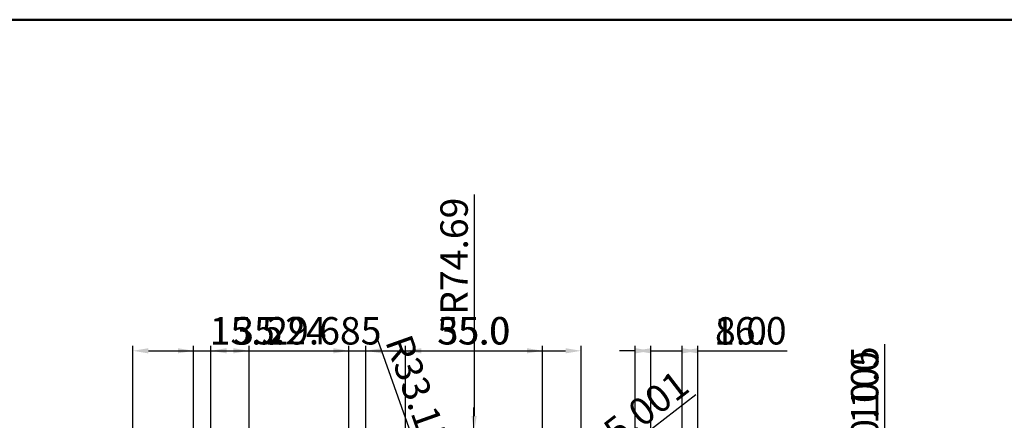
# Model space of a CAD drawing. Units: millimetres. Extents: x -21 to 693, y -570 to 295.
# Tile 6 of 7: x 107 to 359, y 193 to 295. Entities that reach past the tile are written whole.
import ezdxf

# ---------------------------------------------------------------- set-up
doc = ezdxf.new("R2010")
doc.units = ezdxf.units.MM
doc.header["$LTSCALE"] = 0.5
doc.linetypes.add('CENTER2', pattern=[28.575, 19.05, -3.175, 3.175, -3.175])
for name, color, linetype, lineweight in [('M-CNTR', 1, 'CENTER2', 18), ('M-DIMS', 2, 'Continuous', 25), ('M-TTLB', 7, 'Continuous', 50)]:
    doc.layers.add(name, color=color, linetype=linetype, lineweight=lineweight)
doc.styles.get("Standard").update_dxf_attribs({"font": 'arial.ttf'})
doc.dimstyles.new('ISO-25', dxfattribs={"dimtxt": 7, "dimasz": 4, "dimexe": 1.25, "dimexo": 0.625, "dimtad": 1, "dimdec": 0, "dimtxsty": 'Standard', "dimcen": 2.5, "dimadec": 0, "dimazin": 0, "dimtfac": 1, "dimtdec": 0, "dimtofl": 0, "dimtmove": 0, "dimatfit": 3, "dimfxl": 1, "dimarcsym": 0})

# ---------------------------------------------------------------- blocks, each defined once
blk = doc.blocks.new('*D49')
at = {"layer": 'Defpoints', "color": 0, "ltscale": 0.5, "transparency": 16777216}
for p in [(191.43, 210.86), (156.19, 130.11), (191.43, 129.89)]:
    blk.add_point(p, dxfattribs=at)
at = {"layer": 'M-DIMS', "color": 0, "lineweight": -2, "ltscale": 0.5, "transparency": 16777216}
for p, q in [((156.19, 130.74), (156.19, 212.11)), ((191.43, 130.52), (191.43, 212.11)), ((160.19, 210.86), (187.43, 210.86))]:
    blk.add_line(p, q, dxfattribs=at)
at = {"layer": 'M-DIMS', "color": 0, "ltscale": 0.5, "transparency": 16777216}
for points in [[(160.19, 211.53), (160.19, 210.2), (156.19, 210.86)], [(187.43, 211.53), (187.43, 210.2), (191.43, 210.86)]]:
    blk.add_solid(points, dxfattribs=at)
at = {"layer": 'M-DIMS', "color": 0, "ltscale": 0.5, "transparency": 16777216, "insert": (173.81, 215.07), "char_height": 7, "attachment_point": 5}
blk.add_mtext('35.24', dxfattribs=at)
blk = doc.blocks.new('*D52')
at = {"layer": 'Defpoints', "color": 0, "ltscale": 0.5, "transparency": 16777216}
for p in [(151.74, 210.86), (136.24, 115.11), (151.74, 115.11)]:
    blk.add_point(p, dxfattribs=at)
at = {"layer": 'M-DIMS', "color": 0, "lineweight": -2, "ltscale": 0.5, "transparency": 16777216}
for p, q in [((136.24, 115.74), (136.24, 212.11)), ((151.74, 115.74), (151.74, 212.11)), ((140.24, 210.86), (147.74, 210.86)), ((151.74, 210.86), (174.56, 210.86))]:
    blk.add_line(p, q, dxfattribs=at)
at = {"layer": 'M-DIMS', "color": 0, "ltscale": 0.5, "transparency": 16777216}
for points in [[(140.24, 211.53), (140.24, 210.2), (136.24, 210.86)], [(147.74, 211.53), (147.74, 210.2), (151.74, 210.86)]]:
    blk.add_solid(points, dxfattribs=at)
at = {"layer": 'M-DIMS', "color": 0, "ltscale": 0.5, "transparency": 16777216, "insert": (165.15, 215.06), "char_height": 7, "attachment_point": 5}
blk.add_mtext('15.5', dxfattribs=at)
blk = doc.blocks.new('*D56')
at = {"layer": 'Defpoints', "color": 0, "ltscale": 0.5, "transparency": 16777216}
for p in [(165.92, 210.86), (136.24, 148.11), (165.92, 148.11)]:
    blk.add_point(p, dxfattribs=at)
at = {"layer": 'M-DIMS', "color": 0, "lineweight": -2, "ltscale": 0.5, "transparency": 16777216}
for p, q in [((136.24, 148.74), (136.24, 212.11)), ((165.92, 148.74), (165.92, 212.11)), ((140.24, 210.86), (161.92, 210.86)), ((165.92, 210.86), (200.4, 210.86))]:
    blk.add_line(p, q, dxfattribs=at)
at = {"layer": 'M-DIMS', "color": 0, "ltscale": 0.5, "transparency": 16777216}
for points in [[(140.24, 211.53), (140.24, 210.2), (136.24, 210.86)], [(161.92, 211.53), (161.92, 210.2), (165.92, 210.86)]]:
    blk.add_solid(points, dxfattribs=at)
at = {"layer": 'M-DIMS', "color": 0, "ltscale": 0.5, "transparency": 16777216, "insert": (185.16, 215.06), "char_height": 7, "attachment_point": 5}
blk.add_mtext('29.685', dxfattribs=at)
blk = doc.blocks.new('*D57')
at = {"layer": 'Defpoints', "color": 0, "ltscale": 0.5, "transparency": 16777216}
for p in [(280.55, 210.86), (264.55, 135.11), (280.55, 135.11)]:
    blk.add_point(p, dxfattribs=at)
at = {"layer": 'M-DIMS', "color": 0, "lineweight": -2, "ltscale": 0.5, "transparency": 16777216}
for p, q in [((264.55, 135.74), (264.55, 212.11)), ((280.55, 135.74), (280.55, 212.11)), ((268.55, 210.86), (276.55, 210.86)), ((280.55, 210.86), (303.3, 210.86))]:
    blk.add_line(p, q, dxfattribs=at)
at = {"layer": 'M-DIMS', "color": 0, "ltscale": 0.5, "transparency": 16777216}
for points in [[(268.55, 211.53), (268.55, 210.2), (264.55, 210.86)], [(276.55, 211.53), (276.55, 210.2), (280.55, 210.86)]]:
    blk.add_solid(points, dxfattribs=at)
at = {"layer": 'M-DIMS', "color": 0, "ltscale": 0.5, "transparency": 16777216, "insert": (293.93, 215.06), "char_height": 7, "attachment_point": 5}
blk.add_mtext('16.0', dxfattribs=at)
blk = doc.blocks.new('*D59')
at = {"layer": 'Defpoints', "color": 0, "ltscale": 0.5, "transparency": 16777216}
for p in [(276.55, 210.86), (268.55, 153.11), (276.55, 153.11)]:
    blk.add_point(p, dxfattribs=at)
at = {"layer": 'M-DIMS', "color": 0, "lineweight": -2, "ltscale": 0.5, "transparency": 16777216}
for p, q in [((268.55, 153.74), (268.55, 212.11)), ((276.55, 153.74), (276.55, 212.11)), ((264.55, 210.86), (260.55, 210.86)), ((280.55, 210.86), (298.53, 210.86))]:
    blk.add_line(p, q, dxfattribs=at)
at = {"layer": 'M-DIMS', "color": 0, "ltscale": 0.5, "transparency": 16777216}
for points in [[(264.55, 211.53), (264.55, 210.2), (268.55, 210.86)], [(280.55, 211.53), (280.55, 210.2), (276.55, 210.86)]]:
    blk.add_solid(points, dxfattribs=at)
at = {"layer": 'M-DIMS', "color": 0, "ltscale": 0.5, "transparency": 16777216, "insert": (291.54, 215.06), "char_height": 7, "attachment_point": 5}
blk.add_mtext('8.0', dxfattribs=at)
blk = doc.blocks.new('*D61')
at = {"layer": 'Defpoints', "color": 0, "ltscale": 0.5, "transparency": 16777216}
for p in [(250.74, 210.86), (195.74, 173.12), (250.74, 173.32)]:
    blk.add_point(p, dxfattribs=at)
at = {"layer": 'M-DIMS', "color": 0, "lineweight": -2, "ltscale": 0.5, "transparency": 16777216}
for p, q in [((195.74, 173.75), (195.74, 212.11)), ((250.74, 173.95), (250.74, 212.11)), ((199.74, 210.86), (246.74, 210.86))]:
    blk.add_line(p, q, dxfattribs=at)
at = {"layer": 'M-DIMS', "color": 0, "ltscale": 0.5, "transparency": 16777216}
for points in [[(199.74, 211.53), (199.74, 210.2), (195.74, 210.86)], [(246.74, 211.53), (246.74, 210.2), (250.74, 210.86)]]:
    blk.add_solid(points, dxfattribs=at)
at = {"layer": 'M-DIMS', "color": 0, "ltscale": 0.5, "transparency": 16777216, "insert": (223.24, 215.06), "char_height": 7, "attachment_point": 5}
blk.add_mtext('55.0', dxfattribs=at)
blk = doc.blocks.new('*D62')
at = {"layer": 'Defpoints', "color": 0, "ltscale": 0.5, "transparency": 16777216}
for p in [(245.74, 178.22), (328.24, 178.22), (250.74, 148.11)]:
    blk.add_point(p, dxfattribs=at)
at = {"layer": 'M-DIMS', "color": 0, "lineweight": -2, "ltscale": 0.5, "transparency": 16777216}
for p, q in [((328.24, 178.22), (328.24, 212.58)), ((246.36, 178.22), (329.49, 178.22)), ((328.24, 152.11), (328.24, 174.22)), ((251.36, 148.11), (329.49, 148.11))]:
    blk.add_line(p, q, dxfattribs=at)
at = {"layer": 'M-DIMS', "color": 0, "ltscale": 0.5, "transparency": 16777216}
for points in [[(327.57, 174.22), (328.9, 174.22), (328.24, 178.22)], [(327.57, 152.11), (328.9, 152.11), (328.24, 148.11)]]:
    blk.add_solid(points, dxfattribs=at)
at = {"layer": 'M-DIMS', "color": 0, "ltscale": 0.5, "transparency": 16777216, "insert": (324.04, 197.4), "char_height": 7, "attachment_point": 5, "rotation": 90}
blk.add_mtext('30.105', dxfattribs=at)
blk = doc.blocks.new('*D63')
at = {"layer": 'Defpoints', "color": 0, "ltscale": 0.5, "transparency": 16777216}
for p in [(240.89, 210.86), (205.89, 188.11), (240.89, 188.11)]:
    blk.add_point(p, dxfattribs=at)
at = {"layer": 'M-DIMS', "color": 0, "lineweight": -2, "ltscale": 0.5, "transparency": 16777216}
for p, q in [((205.89, 188.74), (205.89, 212.11)), ((240.89, 188.74), (240.89, 212.11)), ((209.89, 210.86), (236.89, 210.86))]:
    blk.add_line(p, q, dxfattribs=at)
at = {"layer": 'M-DIMS', "color": 0, "ltscale": 0.5, "transparency": 16777216}
for points in [[(209.89, 211.53), (209.89, 210.2), (205.89, 210.86)], [(236.89, 211.53), (236.89, 210.2), (240.89, 210.86)]]:
    blk.add_solid(points, dxfattribs=at)
at = {"layer": 'M-DIMS', "color": 0, "ltscale": 0.5, "transparency": 16777216, "insert": (223.39, 215.07), "char_height": 7, "attachment_point": 5}
blk.add_mtext('35.0', dxfattribs=at)
blk = doc.blocks.new('*D64')
at = {"layer": 'Defpoints', "color": 0, "ltscale": 0.5, "transparency": 16777216}
for p in [(240.89, 188.11), (328.24, 188.11), (240.89, 178.11)]:
    blk.add_point(p, dxfattribs=at)
at = {"layer": 'M-DIMS', "color": 0, "lineweight": -2, "ltscale": 0.5, "transparency": 16777216}
for p, q in [((328.24, 188.11), (328.24, 210.86)), ((241.51, 188.11), (329.49, 188.11)), ((328.24, 182.11), (328.24, 184.11)), ((241.51, 178.11), (329.49, 178.11))]:
    blk.add_line(p, q, dxfattribs=at)
at = {"layer": 'M-DIMS', "color": 0, "ltscale": 0.5, "transparency": 16777216}
for points in [[(327.57, 184.11), (328.9, 184.11), (328.24, 188.11)], [(327.57, 182.11), (328.9, 182.11), (328.24, 178.11)]]:
    blk.add_solid(points, dxfattribs=at)
at = {"layer": 'M-DIMS', "color": 0, "ltscale": 0.5, "transparency": 16777216, "insert": (324.04, 201.49), "char_height": 7, "attachment_point": 5, "rotation": 90}
blk.add_mtext('10.0', dxfattribs=at)
blk = doc.blocks.new('*D69')
at = {"layer": 'Defpoints', "color": 0, "ltscale": 0.5, "transparency": 16777216}
for p in [(249.7, 176.27), (245.74, 173.22)]:
    blk.add_point(p, dxfattribs=at)
at = {"layer": 'M-DIMS', "color": 0, "lineweight": -2, "ltscale": 0.5, "transparency": 16777216}
for p, q in [((279.98, 199.59), (252.87, 178.71)), ((245.74, 170.72), (245.74, 175.72)), ((243.24, 173.22), (248.24, 173.22))]:
    blk.add_line(p, q, dxfattribs=at)
at = {"layer": 'M-DIMS', "color": 0, "ltscale": 0.5, "transparency": 16777216}
blk.add_solid([(252.46, 179.24), (253.28, 178.18), (249.7, 176.27)], dxfattribs=at)
at = {"layer": 'M-DIMS', "color": 0, "ltscale": 0.5, "transparency": 16777216, "insert": (265.45, 193.7), "char_height": 7, "attachment_point": 5, "rotation": 37.6005}
blk.add_mtext('R5.001', dxfattribs=at)
blk = doc.blocks.new('*D70')
at = {"layer": 'Defpoints', "color": 0, "ltscale": 0.5, "transparency": 16777216}
for p in [(212.11, 176.19), (223.23, 144.96)]:
    blk.add_point(p, dxfattribs=at)
at = {"layer": 'M-DIMS', "color": 0, "lineweight": -2, "ltscale": 0.5, "transparency": 16777216}
for p, q in [((198.82, 213.52), (210.77, 179.96)), ((223.23, 142.46), (223.23, 147.46)), ((220.73, 144.96), (225.73, 144.96))]:
    blk.add_line(p, q, dxfattribs=at)
at = {"layer": 'M-DIMS', "color": 0, "ltscale": 0.5, "transparency": 16777216}
blk.add_solid([(211.4, 180.18), (210.14, 179.74), (212.11, 176.19)], dxfattribs=at)
at = {"layer": 'M-DIMS', "color": 0, "ltscale": 0.5, "transparency": 16777216, "insert": (208.08, 200.03), "char_height": 7, "attachment_point": 5, "rotation": 289.5972}
blk.add_mtext('R33.15', dxfattribs=at)
blk = doc.blocks.new('*D71')
at = {"layer": 'Defpoints', "color": 0, "ltscale": 0.5, "transparency": 16777216}
for p in [(223.39, 190.19), (223.39, 115.5)]:
    blk.add_point(p, dxfattribs=at)
at = {"layer": 'M-DIMS', "color": 0, "lineweight": -2, "ltscale": 0.5, "transparency": 16777216}
for p, q in [((223.39, 250.8), (223.39, 194.19)), ((223.39, 113), (223.39, 118)), ((220.89, 115.5), (225.89, 115.5))]:
    blk.add_line(p, q, dxfattribs=at)
at = {"layer": 'M-DIMS', "color": 0, "ltscale": 0.5, "transparency": 16777216}
blk.add_solid([(222.72, 194.19), (224.06, 194.19), (223.39, 190.19)], dxfattribs=at)
at = {"layer": 'M-DIMS', "color": 0, "ltscale": 0.5, "transparency": 16777216, "insert": (219.19, 235.01), "char_height": 7, "attachment_point": 5, "rotation": 89.9979}
blk.add_mtext('R74.69', dxfattribs=at)

msp = doc.modelspace()

# ---------------------------------------------------------------- linework, layer by layer
at = {"layer": 'M-CNTR'}
msp.add_line((223.2368, 148.1134), (223.2368, 196.364), dxfattribs=at)
at = {"layer": 'M-TTLB', "ltscale": 0.5}
msp.add_lwpolyline([(-21.49, 295.4176), (693.1139, 295.4176), (693.1139, -570.0874), (-21.49, -570.0874)], close=True, dxfattribs=at)

# ---------------------------------------------------------------- dimensions: what is measured, and where the dimension line sits
at = {"layer": 'M-DIMS', "ltscale": 0.5}
dim = msp.add_radius_dim(center=(223.3872, 115.5045), mpoint=(223.39, 190.1925), dimstyle='ISO-25', override={"dimdec": 2, "dimlfac": 1, "dimrnd": 0, "dimzin": 0, "dimdsep": 46, "dimlunit": 2}, dxfattribs=at)
dim.commit()
dim.dimension.update_dxf_attribs({"geometry": '*D71', "text_midpoint": (223.3917, 235.0053), "dimtype": 164})
for base, p1, p2, override, picture, middle in [((151.7368, 210.864), (136.2368, 115.1134), (151.7368, 115.1134), {"dimdec": 1, "dimlfac": 1, "dimrnd": 0, "dimzin": 0, "dimdsep": 46, "dimlunit": 2}, '*D52', (165.15, 215.063)), ((165.9215, 210.864), (136.2368, 148.1134), (165.9215, 148.1134), {"dimdec": 3, "dimlfac": 1, "dimrnd": 0, "dimzin": 0, "dimdsep": 46, "dimlunit": 2}, '*D56', (185.1625, 215.063)), ((191.4283, 210.864), (156.1864, 130.1134), (191.4283, 129.8948), {"dimdec": 2, "dimlfac": 1, "dimrnd": 0, "dimzin": 0, "dimdsep": 46, "dimlunit": 2}, '*D49', (173.8073, 215.0654)), ((250.7368, 210.864), (195.7368, 173.1232), (250.7368, 173.3203), {"dimdec": 1, "dimlfac": 1, "dimrnd": 0, "dimzin": 0, "dimdsep": 46, "dimlunit": 2}, '*D61', (223.2368, 215.063)), ((240.8872, 210.864), (205.8872, 188.1134), (240.8872, 188.1134), {"dimdec": 1, "dimlfac": 1, "dimrnd": 0, "dimzin": 0, "dimdsep": 46, "dimlunit": 2}, '*D63', (223.3872, 215.0654)), ((276.5522, 210.864), (268.5522, 153.1134), (276.5522, 153.1134), {"dimdec": 1, "dimlfac": 1, "dimrnd": 0, "dimzin": 0, "dimdsep": 46, "dimlunit": 2}, '*D59', (291.5421, 215.063)), ((280.5522, 210.864), (264.5522, 135.1134), (280.5522, 135.1134), {"dimdec": 1, "dimlfac": 1, "dimrnd": 0, "dimzin": 0, "dimdsep": 46, "dimlunit": 2}, '*D57', (293.9272, 215.063))]:
    dim = msp.add_linear_dim(base=base, p1=p1, p2=p2, dimstyle='ISO-25', override=override, dxfattribs=at)
    dim.commit()
    dim.dimension.update_dxf_attribs({"geometry": picture, "text_midpoint": middle})
for center, mpoint, override, picture, middle in [((223.2289, 144.9606), (212.1093, 176.193), {"dimdec": 2, "dimlfac": 1, "dimrnd": 0, "dimzin": 0, "dimdsep": 46, "dimlunit": 2}, '*D70', (208.0808, 200.0344)), ((245.7368, 173.2169), (249.6991, 176.2683), {"dimdec": 3, "dimlfac": 1, "dimrnd": 0, "dimzin": 0, "dimdsep": 46, "dimlunit": 2}, '*D69', (265.4465, 193.6955))]:
    dim = msp.add_radius_dim(center=center, mpoint=mpoint, dimstyle='ISO-25', override=override, dxfattribs=at)
    dim.commit()
    dim.dimension.update_dxf_attribs({"geometry": picture, "text_midpoint": middle})
for base, p1, p2, override, picture, middle in [((328.23683, 178.21793), (250.73683, 148.11336), (245.73683, 178.21793), {"dimdec": 3, "dimlfac": 1, "dimrnd": 0, "dimzin": 0, "dimdsep": 46, "dimlunit": 2}, '*D62', (324.03543, 197.39682)), ((328.2368, 188.1134), (240.8872, 178.1134), (240.8872, 188.1134), {"dimdec": 1, "dimlfac": 1, "dimrnd": 0, "dimzin": 0, "dimdsep": 46, "dimlunit": 2}, '*D64', (324.0378, 201.4884))]:
    dim = msp.add_linear_dim(base=base, p1=p1, p2=p2, angle=90, dimstyle='ISO-25', override=override, dxfattribs=at)
    dim.commit()
    dim.dimension.update_dxf_attribs({"geometry": picture, "text_midpoint": middle})

doc.saveas('drawing.dxf')
